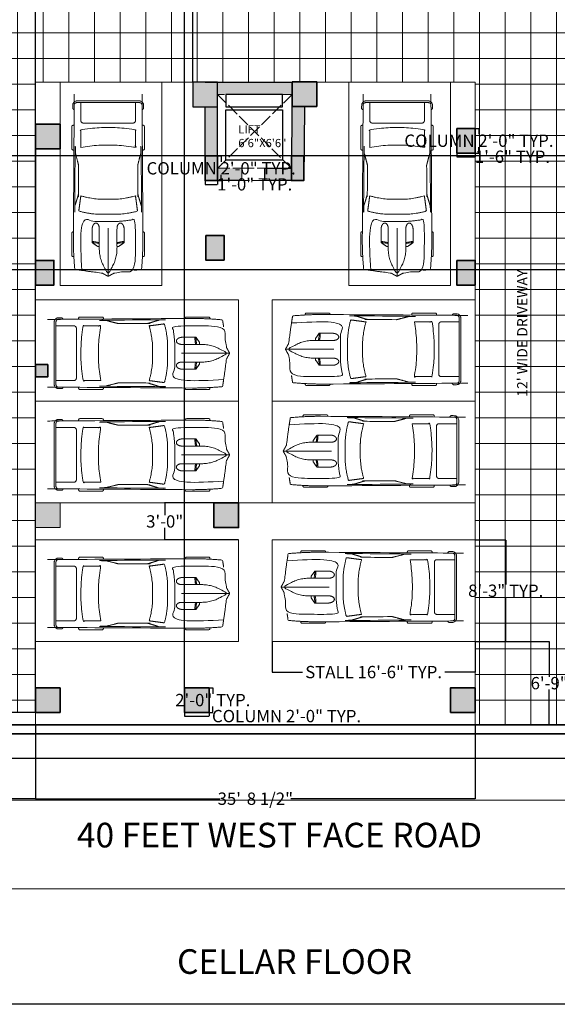
# Model space of a CAD drawing. Units: inches. Extents: x 48986 to 50522, y 132527 to 134098.
# Tile 2 of 4: x 49552 to 50076, y 132529 to 133488. Entities that reach past the tile are written whole.
import ezdxf

# ---------------------------------------------------------------- set-up
doc = ezdxf.new("R2010")
doc.units = ezdxf.units.IN
doc.header["$MEASUREMENT"] = 0
doc.linetypes.add('ACAD_ISO02W100', pattern=[15, 12, -3])
for name, color, linetype, lineweight in [('A-ANNO-DIMS', 2, 'Continuous', 18), ('A-ANNO-TEXT', 7, 'Continuous', 18), ('A-ANNO-TTLB', 7, 'Continuous', 25), ('A-AREA-IDEN', 7, 'Continuous', 18), ('A-COLS-PATT', 215, 'Continuous', 13), ('A-EQPM-VEHC', 8, 'Continuous', 13), ('A-FLOR-EVTR', 7, 'Continuous', 25), ('A-FLOR-PATT', 94, 'Continuous', 9), ('A-FLOR-PKNG', 140, 'Continuous', 18), ('A-WALL-PATT', 254, 'Continuous', 13), ('C-PROP', 160, 'Continuous', 25), ('C-ROAD', 7, 'Continuous', 18), ('COLUMNS', 211, 'Continuous', 35), ('lift', 7, 'ACAD_ISO02W100', 18), ('WALLS', 140, 'Continuous', 35)]:
    doc.layers.add(name, color=color, linetype=linetype, lineweight=lineweight)
doc.styles.get("Standard").update_dxf_attribs({"font": 'arial.ttf'})
doc.dimstyles.get("Standard").update_dxf_attribs({"dimtxt": 12, "dimasz": 0.18, "dimexe": 0.18, "dimexo": 0.0625, "dimgap": 0.09, "dimtad": 0, "dimtih": 1, "dimtoh": 1, "dimdec": 1, "dimzin": 0, "dimdsep": 46, "dimlunit": 3, "dimtxsty": 'Standard', "dimcen": 0.09, "dimadec": 0, "dimazin": 0, "dimtfac": 1, "dimtdec": 1, "dimtofl": 0, "dimtmove": 0, "dimatfit": 3, "dimfxl": 1, "dimtolj": 1, "dimtzin": 0, "dimarcsym": 0})

# ---------------------------------------------------------------- blocks, each defined once
blk = doc.blocks.new('CAR-SEDAN-PLAN')
for p, q in [((35.28, 177.53), (35.28, 130.65)), ((25.73, 8.37), (44.83, 8.37))]:
    blk.add_line(p, q)
for centre, major_axis, start_param, end_param in [((19.85, 164.65), (-24.87, 0), 1.564964, 1.848039), ((50.71, 164.65), (24.87, 0), 4.435146, 4.718221)]:
    blk.add_ellipse(centre, major_axis=major_axis, ratio=0.842304, start_param=start_param, end_param=end_param)
for points, weights, knots in [([(60.93, 171.77), (56.4, 172.48), (51.85, 173.06), (46.33, 173.7), (40.84, 174.57), (38.25, 176), (35.65, 177.44), (35.28, 177.64), (34.91, 177.44), (32.32, 176), (29.72, 174.57), (24.24, 173.7), (18.71, 173.06), (14.16, 172.48), (9.64, 171.77), (7.88, 146.82), (9.23, 121.85), (17.23, 123.66), (25.51, 124.08), (35.28, 124.08), (45.06, 124.08), (53.33, 123.66), (61.34, 121.85), (62.69, 146.82), (60.93, 171.77)], [1, 0.999861960732, 1, 0.999699858145, 1, 1, 1, 0.835952709181, 1, 1, 1, 0.999699858145, 1, 0.999861960732, 1, 0.998625728423, 1, 0.994860280211, 1, 1, 1, 0.994860280211, 1, 0.998625728423, 1], [0, 0, 0, 0.033232, 0.033232, 0.082234, 0.082234, 1.082234, 1.082234, 2.244094, 2.244094, 3.244094, 3.244094, 3.293097, 3.293097, 3.326328, 3.326328, 3.431193, 3.431193, 3.634055, 3.634055, 4.634055, 4.634055, 4.836917, 4.836917, 4.941783, 4.941783, 4.941783]), ([(43.91, 145.56), (47.31, 144.74), (50.86, 144.76), (50.86, 138.04), (50.86, 131.32), (50.59, 126.02), (47.38, 125.71), (44.17, 125.4), (43.91, 130.65), (43.91, 140.58), (43.91, 150.52), (43.91, 163.57), (35.28, 174.41), (26.66, 163.57), (26.66, 150.52), (26.66, 140.58), (26.66, 130.65), (26.39, 125.4), (23.18, 125.71), (19.97, 126.02), (19.71, 131.32), (19.71, 138.04), (19.71, 144.76), (23.25, 144.74), (26.66, 145.56)], [1, 0.990000279832, 1, 1, 1, 0.735618766318, 1, 0.735618766318, 1, 1, 1, 0.956755789522, 1, 0.956755789522, 1, 1, 1, 0.735618766318, 1, 0.735618766318, 1, 1, 1, 0.990000279832, 1], [0, 0, 0, 0.283075, 0.283075, 1.283075, 1.283075, 2.771508, 2.771508, 4.259942, 4.259942, 5.259942, 5.259942, 5.85026, 5.85026, 6.440579, 6.440579, 7.440579, 7.440579, 8.929012, 8.929012, 10.417446, 10.417446, 11.417446, 11.417446, 11.700521, 11.700521, 11.700521]), ([(9.64, 171.77), (6.18, 171.25), (2.75, 170.65), (1.43, 155.99), (1.38, 141.3)], [1, 0.999923835344, 1, 0.999337806115, 1], [0, 0, 0, 0.02468451, 0.02468451, 0.0974728, 0.0974728, 0.0974728]), ([(69.18, 141.3), (69.13, 155.99), (67.82, 170.65), (64.38, 171.25), (60.93, 171.77)], [1, 0.999337806115, 1, 0.999923835344, 1], [0, 0, 0, 0.07278829, 0.07278829, 0.0974728, 0.0974728, 0.0974728]), ([(1.87, 158.39), (1.61, 158.39), (1.35, 158.39), (0.79, 158.39), (0.4, 158.06), (0, 157.72), (0, 157.26), (0, 146.28), (0, 135.3), (0, 134.83), (0.4, 134.5), (0.79, 134.17), (1.35, 134.17), (1.35, 134.17), (1.36, 134.17)], [1, 1, 1, 0.923879532511, 1, 0.923879532511, 1, 1, 1, 0.923879532511, 1, 0.923879532511, 1, 1, 1], [0, 0, 0, 1, 1, 1.785398, 1.785398, 2.570796, 2.570796, 3.570796, 3.570796, 4.356194, 4.356194, 5.141593, 5.141593, 6.141593, 6.141593, 6.141593]), ([(69.2, 134.17), (69.21, 134.17), (69.22, 134.17), (69.77, 134.17), (70.17, 134.5), (70.56, 134.83), (70.56, 135.3), (70.56, 146.28), (70.56, 157.26), (70.56, 157.72), (70.17, 158.06), (69.77, 158.39), (69.22, 158.39), (68.96, 158.39), (68.7, 158.39)], [1, 1, 1, 0.923879532511, 1, 0.923879532511, 1, 1, 1, 0.923879532511, 1, 0.923879532511, 1, 1, 1], [0, 0, 0, 1, 1, 1.785398, 1.785398, 2.570796, 2.570796, 3.570796, 3.570796, 4.356194, 4.356194, 5.141593, 5.141593, 6.141593, 6.141593, 6.141593]), ([(26.66, 148.39), (25.91, 148.39), (25.16, 148.39), (24.92, 148.39), (24.74, 148.26), (22.22, 146.51), (19.71, 144.76)], [1, 1, 1, 0.940892222322, 1, 1, 1], [0, 0, 0, 1, 1, 1.691083, 1.691083, 2.691083, 2.691083, 2.691083]), ([(50.86, 144.76), (48.34, 146.51), (45.83, 148.26), (45.64, 148.39), (45.4, 148.39), (44.65, 148.39), (43.91, 148.39)], [1, 1, 1, 0.940892222322, 1, 1, 1], [0, 0, 0, 1, 1, 1.691083, 1.691083, 2.691083, 2.691083, 2.691083]), ([(1.38, 141.68), (1.17, 76.13), (2.21, 10.6), (2.24, 8.37), (4.89, 8.37), (35.28, 8.37), (65.67, 8.37), (68.32, 8.37), (68.36, 10.6), (69.4, 76.13), (69.18, 141.68)], [1, 0.999967219517, 1, 0.711827418646, 1, 1, 1, 0.711827418646, 1, 0.999967219517, 1], [0, 0, 0, 0.016194, 0.016194, 1.573593, 1.573593, 2.573593, 2.573593, 4.130993, 4.130993, 4.147187, 4.147187, 4.147187]), ([(6.45, 69.32), (4.72, 62.5), (2.98, 55.69), (2.73, 82.7), (2.7, 109.71), (4.53, 103.71), (6.37, 97.71), (6.33, 83.51), (6.45, 69.32)], [1, 1, 1, 0.999994429546, 1, 1, 1, 0.999987377106, 1], [0, 0, 0, 1, 1, 1.006676, 1.006676, 2.006676, 2.006676, 2.016725, 2.016725, 2.016725]), ([(61.91, 99.15), (52.72, 101.89), (42.99, 102.47), (35.28, 102.47), (27.57, 102.47), (17.85, 101.89), (8.66, 99.15), (7.66, 106.57), (6.67, 114), (15.95, 116.64), (25.73, 117.16), (35.28, 117.16), (44.83, 117.16), (54.61, 116.64), (63.89, 114), (62.9, 106.57), (61.91, 99.15)], [1, 0.991000078903, 1, 1, 1, 0.991000078903, 1, 1, 1, 0.991394232237, 1, 1, 1, 0.991394232237, 1, 1, 1], [0, 0, 0, 0.268529, 0.268529, 1.268529, 1.268529, 1.537057, 1.537057, 2.537057, 2.537057, 2.799631, 2.799631, 3.799631, 3.799631, 4.062205, 4.062205, 5.062205, 5.062205, 5.062205]), ([(64.11, 69.32), (64.24, 83.51), (64.2, 97.71), (66.03, 103.71), (67.87, 109.71), (67.83, 82.7), (67.58, 55.69), (65.85, 62.5), (64.11, 69.32)], [1, 0.999987377106, 1, 1, 1, 0.999994429546, 1, 1, 1], [0, 0, 0, 0.010049, 0.010049, 1.010049, 1.010049, 1.016725, 1.016725, 2.016725, 2.016725, 2.016725]), ([(1.65, 54.65), (1.5, 54.65), (1.35, 54.65), (0, 54.65), (0, 53.52), (0, 42.54), (0, 31.57), (0, 30.44), (1.35, 30.44), (1.63, 30.44), (1.92, 30.44)], [1, 1, 1, 0.707106781187, 1, 1, 1, 0.707106781187, 1, 1, 1], [0, 0, 0, 1, 1, 2.570796, 2.570796, 3.570796, 3.570796, 5.141593, 5.141593, 6.141593, 6.141593, 6.141593]), ([(61.91, 51.96), (35.28, 47.39), (8.66, 51.96), (8.66, 43.42), (8.66, 34.88), (35.28, 30.31), (61.91, 34.88), (61.91, 43.42), (61.91, 51.96)], [1, 0.979868494456, 1, 1, 1, 0.979868494456, 1, 1, 1], [0, 0, 0, 0.401989, 0.401989, 1.401989, 1.401989, 1.803978, 1.803978, 2.803978, 2.803978, 2.803978]), ([(68.64, 30.44), (68.93, 30.44), (69.22, 30.44), (69.77, 30.44), (70.17, 30.77), (70.56, 31.1), (70.56, 31.57), (70.56, 42.54), (70.56, 53.52), (70.56, 53.99), (70.17, 54.32), (69.77, 54.65), (69.22, 54.65), (69.07, 54.65), (68.91, 54.65)], [1, 1, 1, 0.923879532511, 1, 0.923879532511, 1, 1, 1, 0.923879532511, 1, 0.923879532511, 1, 1, 1], [0, 0, 0, 1, 1, 1.785398, 1.785398, 2.570796, 2.570796, 3.570796, 3.570796, 4.356194, 4.356194, 5.141593, 5.141593, 6.141593, 6.141593, 6.141593]), ([(61.91, 8.37), (61.91, 17.2), (61.91, 26.03), (61.91, 28.29), (59.22, 28.29), (35.28, 28.29), (11.34, 28.29), (8.66, 28.29), (8.66, 26.03), (8.66, 17.2), (8.66, 8.37)], [1, 1, 1, 0.707106781187, 1, 1, 1, 0.707106781187, 1, 1, 1], [0, 0, 0, 1, 1, 2.570796, 2.570796, 3.570796, 3.570796, 5.141593, 5.141593, 6.141593, 6.141593, 6.141593]), ([(2.14, 15.28), (0.74, 14.89), (0.76, 13.65), (0.78, 12.11), (0.81, 10.58), (0.87, 6.62), (5.56, 6.62), (35.28, 6.62), (65, 6.62), (69.7, 6.62), (69.76, 10.58), (69.78, 12.11), (69.81, 13.65), (69.83, 14.89), (68.43, 15.28)], [1, 0.807168985933, 1, 0.999999981995, 1, 0.711827418646, 1, 1, 1, 0.711827418646, 1, 0.999999981995, 1, 0.807168985459, 1], [0, 0, 0, 1.262912, 1.262912, 1.263291, 1.263291, 2.82069, 2.82069, 3.82069, 3.82069, 5.37809, 5.37809, 5.378469, 5.378469, 6.641381, 6.641381, 6.641381])]:
    blk.add_rational_spline(points, weights, degree=2, knots=knots)
blk = doc.blocks.new('PARKING-STALL-99X198')
blk.add_lwpolyline([(198, 0), (198, 99), (0, 99), (0, 0)], close=True)
blk = doc.blocks.new('COL-24X24')
blk.add_lwpolyline([(24, 24), (24, 0), (0, 0), (0, 24)], close=True)
blk = doc.blocks.new('COL-18X24')
blk.add_lwpolyline([(0, 24), (0, 12.32), (0, 0), (18, 0), (18, 24)], close=True)
blk = doc.blocks.new('COL-12X24')
blk.add_lwpolyline([(0, 24), (12, 24), (12, 0), (0, 0)], close=True)
blk = doc.blocks.new('*D13')
at = {"layer": 'A-ANNO-DIMS', "color": 0, "lineweight": -2, "transparency": 16777216}
for p, q in [((49797.88, 132881.98), (49797.88, 132852.17)), ((49995.88, 132881.98), (49995.88, 132852.17)), ((49798.06, 132852.35), (49827.63, 132852.35)), ((49995.7, 132852.35), (49966.13, 132852.35))]:
    blk.add_line(p, q, dxfattribs=at)
at = {"layer": 'A-ANNO-DIMS', "color": 0, "transparency": 16777216}
for points in [[(49798.06, 132852.38), (49798.06, 132852.32), (49797.88, 132852.35)], [(49995.7, 132852.38), (49995.7, 132852.32), (49995.88, 132852.35)]]:
    blk.add_solid(points, dxfattribs=at)
at = {"layer": 'Defpoints', "color": 0, "transparency": 16777216}
for p in [(49797.88, 132882.05), (49995.88, 132882.05), (49995.88, 132852.35)]:
    blk.add_point(p, dxfattribs=at)
at = {"layer": 'A-ANNO-DIMS', "color": 0, "transparency": 16777216, "insert": (49896.88, 132852.35), "char_height": 12, "attachment_point": 5}
blk.add_mtext('\\A1;STALL 16\'-6" TYP.', dxfattribs=at)
blk = doc.blocks.new('*D14')
at = {"layer": 'A-ANNO-DIMS', "color": 0, "lineweight": -2, "transparency": 16777216}
for p, q in [((49995.94, 132981.05), (50025.76, 132981.05)), ((50025.58, 132980.87), (50025.58, 132937.77)), ((50025.58, 132882.23), (50025.58, 132925.32)), ((49995.94, 132882.05), (50025.76, 132882.05))]:
    blk.add_line(p, q, dxfattribs=at)
at = {"layer": 'A-ANNO-DIMS', "color": 0, "transparency": 16777216}
for points in [[(50025.55, 132980.87), (50025.61, 132980.87), (50025.58, 132981.05)], [(50025.55, 132882.23), (50025.61, 132882.23), (50025.58, 132882.05)]]:
    blk.add_solid(points, dxfattribs=at)
at = {"layer": 'Defpoints', "color": 0, "transparency": 16777216}
for p in [(49995.88, 132981.05), (50025.58, 132981.05), (49995.88, 132882.05)]:
    blk.add_point(p, dxfattribs=at)
at = {"layer": 'A-ANNO-DIMS', "color": 0, "transparency": 16777216, "insert": (50025.58, 132931.55), "char_height": 12, "attachment_point": 5}
blk.add_mtext('\\A1;8\'-3" TYP.', dxfattribs=at)
blk = doc.blocks.new('*D15')
at = {"layer": 'A-ANNO-DIMS', "color": 0, "lineweight": -2, "transparency": 16777216}
for p, q in [((49712.57, 132812.99), (49712.57, 132809.28)), ((49712.75, 132809.46), (49736.39, 132809.46)), ((49736.57, 132812.99), (49736.57, 132809.28)), ((49736.57, 132809.46), (49736.75, 132809.46))]:
    blk.add_line(p, q, dxfattribs=at)
at = {"layer": 'A-ANNO-DIMS', "color": 0, "transparency": 16777216}
for points in [[(49712.75, 132809.49), (49712.75, 132809.43), (49712.57, 132809.46)], [(49736.39, 132809.49), (49736.39, 132809.43), (49736.57, 132809.46)]]:
    blk.add_solid(points, dxfattribs=at)
at = {"layer": 'Defpoints', "color": 0, "transparency": 16777216}
for p in [(49712.57, 132813.06), (49736.57, 132813.06), (49736.57, 132809.46)]:
    blk.add_point(p, dxfattribs=at)
at = {"layer": 'A-ANNO-DIMS', "color": 0, "transparency": 16777216, "insert": (49812, 132809.46), "char_height": 12, "attachment_point": 5}
blk.add_mtext('\\A1;COLUMN 2\'-0" TYP.', dxfattribs=at)
blk = doc.blocks.new('*D16')
at = {"layer": 'A-ANNO-DIMS', "color": 0, "lineweight": -2, "transparency": 16777216}
for p, q in [((49736.63, 132837.06), (49740.35, 132837.06)), ((49740.17, 132836.88), (49740.17, 132831.27)), ((49740.17, 132813.24), (49740.17, 132818.84)), ((49736.63, 132813.06), (49740.35, 132813.06))]:
    blk.add_line(p, q, dxfattribs=at)
at = {"layer": 'A-ANNO-DIMS', "color": 0, "transparency": 16777216}
for points in [[(49740.14, 132836.88), (49740.2, 132836.88), (49740.17, 132837.06)], [(49740.14, 132813.24), (49740.2, 132813.24), (49740.17, 132813.06)]]:
    blk.add_solid(points, dxfattribs=at)
at = {"layer": 'Defpoints', "color": 0, "transparency": 16777216}
for p in [(49736.57, 132837.06), (49740.17, 132837.06), (49736.57, 132813.06)]:
    blk.add_point(p, dxfattribs=at)
at = {"layer": 'A-ANNO-DIMS', "color": 0, "transparency": 16777216, "insert": (49740.17, 132825.06), "char_height": 12, "attachment_point": 5}
blk.add_mtext('\\A1;2\'-0" TYP.', dxfattribs=at)
blk = doc.blocks.new('*D17')
at = {"layer": 'A-ANNO-DIMS', "color": 0, "lineweight": -2, "transparency": 16777216}
for p, q in [((49995.94, 133381.91), (49999.66, 133381.91)), ((49999.48, 133381.73), (49999.48, 133376.2)), ((49999.48, 133358.09), (49999.48, 133363.61)), ((49995.94, 133357.91), (49999.66, 133357.91))]:
    blk.add_line(p, q, dxfattribs=at)
at = {"layer": 'A-ANNO-DIMS', "color": 0, "transparency": 16777216}
for points in [[(49999.45, 133381.73), (49999.51, 133381.73), (49999.48, 133381.91)], [(49999.45, 133358.09), (49999.51, 133358.09), (49999.48, 133357.91)]]:
    blk.add_solid(points, dxfattribs=at)
at = {"layer": 'Defpoints', "color": 0, "transparency": 16777216}
for p in [(49995.88, 133381.91), (49999.48, 133381.91), (49995.88, 133357.91)]:
    blk.add_point(p, dxfattribs=at)
at = {"layer": 'A-ANNO-DIMS', "color": 0, "transparency": 16777216, "insert": (49999.48, 133369.91), "char_height": 12, "attachment_point": 5}
blk.add_mtext('\\A1;COLUMN 2\'-0" TYP.', dxfattribs=at)
blk = doc.blocks.new('*D18')
at = {"layer": 'A-ANNO-DIMS', "color": 0, "lineweight": -2, "transparency": 16777216}
for p, q in [((49977.88, 133357.84), (49977.88, 133354.13)), ((49978.06, 133354.31), (49995.7, 133354.31)), ((49995.88, 133357.84), (49995.88, 133354.13)), ((49995.88, 133354.31), (49996.06, 133354.31))]:
    blk.add_line(p, q, dxfattribs=at)
at = {"layer": 'A-ANNO-DIMS', "color": 0, "transparency": 16777216}
for points in [[(49978.06, 133354.34), (49978.06, 133354.28), (49977.88, 133354.31)], [(49995.7, 133354.34), (49995.7, 133354.28), (49995.88, 133354.31)]]:
    blk.add_solid(points, dxfattribs=at)
at = {"layer": 'Defpoints', "color": 0, "transparency": 16777216}
for p in [(49977.88, 133357.91), (49995.88, 133357.91), (49995.88, 133354.31)]:
    blk.add_point(p, dxfattribs=at)
at = {"layer": 'A-ANNO-DIMS', "color": 0, "transparency": 16777216, "insert": (50032.16, 133354.31), "char_height": 12, "attachment_point": 5}
blk.add_mtext('\\A1;1\'-6" TYP.', dxfattribs=at)
blk = doc.blocks.new('*D21')
at = {"layer": 'A-ANNO-DIMS', "color": 0, "lineweight": -2, "transparency": 16777216}
for p, q in [((49744.77, 133355), (49748.49, 133355)), ((49748.31, 133354.82), (49748.31, 133349.3)), ((49748.31, 133331.18), (49748.31, 133336.7)), ((49744.77, 133331), (49748.49, 133331))]:
    blk.add_line(p, q, dxfattribs=at)
at = {"layer": 'A-ANNO-DIMS', "color": 0, "transparency": 16777216}
for points in [[(49748.28, 133354.82), (49748.34, 133354.82), (49748.31, 133355)], [(49748.28, 133331.18), (49748.34, 133331.18), (49748.31, 133331)]]:
    blk.add_solid(points, dxfattribs=at)
at = {"layer": 'Defpoints', "color": 0, "transparency": 16777216}
for p in [(49744.71, 133355), (49748.31, 133355), (49744.71, 133331)]:
    blk.add_point(p, dxfattribs=at)
at = {"layer": 'A-ANNO-DIMS', "color": 0, "transparency": 16777216, "insert": (49748.31, 133343), "char_height": 12, "attachment_point": 5}
blk.add_mtext('\\A1;COLUMN 2\'-0" TYP.', dxfattribs=at)
blk = doc.blocks.new('*D22')
at = {"layer": 'A-ANNO-DIMS', "color": 0, "lineweight": -2, "transparency": 16777216}
for p, q in [((49732.71, 133330.93), (49732.71, 133327.22)), ((49732.89, 133327.4), (49744.53, 133327.4)), ((49744.71, 133330.93), (49744.71, 133327.22)), ((49744.71, 133327.4), (49744.89, 133327.4))]:
    blk.add_line(p, q, dxfattribs=at)
at = {"layer": 'A-ANNO-DIMS', "color": 0, "transparency": 16777216}
for points in [[(49732.89, 133327.43), (49732.89, 133327.37), (49732.71, 133327.4)], [(49744.53, 133327.43), (49744.53, 133327.37), (49744.71, 133327.4)]]:
    blk.add_solid(points, dxfattribs=at)
at = {"layer": 'Defpoints', "color": 0, "transparency": 16777216}
for p in [(49732.71, 133331), (49744.71, 133331), (49744.71, 133327.4)]:
    blk.add_point(p, dxfattribs=at)
at = {"layer": 'A-ANNO-DIMS', "color": 0, "transparency": 16777216, "insert": (49780.99, 133327.4), "char_height": 12, "attachment_point": 5}
blk.add_mtext('\\A1;1\'-0" TYP.', dxfattribs=at)
blk = doc.blocks.new('*D27')
at = {"layer": 'A-ANNO-DIMS', "color": 0, "lineweight": -2, "transparency": 16777216}
for p, q in [((49221.79, 132800.99), (49221.79, 132728.83)), ((49567.36, 132800.99), (49567.36, 132728.83)), ((49221.97, 132729.01), (49359.79, 132729.01)), ((49567.18, 132729.01), (49429.36, 132729.01))]:
    blk.add_line(p, q, dxfattribs=at)
at = {"layer": 'A-ANNO-DIMS', "color": 0, "transparency": 16777216}
for points in [[(49221.97, 132729.04), (49221.97, 132728.98), (49221.79, 132729.01)], [(49567.18, 132729.04), (49567.18, 132728.98), (49567.36, 132729.01)]]:
    blk.add_solid(points, dxfattribs=at)
at = {"layer": 'Defpoints', "color": 0, "transparency": 16777216}
for p in [(49221.79, 132801.06), (49567.36, 132801.06), (49221.79, 132729.01)]:
    blk.add_point(p, dxfattribs=at)
at = {"layer": 'A-ANNO-DIMS', "color": 0, "transparency": 16777216, "insert": (49394.57, 132729.01), "char_height": 12, "attachment_point": 5}
blk.add_mtext('\\A1;28\'-9 1/2"', dxfattribs=at)
blk = doc.blocks.new('*D28')
at = {"layer": 'A-ANNO-DIMS', "color": 0, "lineweight": -2, "transparency": 16777216}
for p, q in [((49567.36, 132800.99), (49567.36, 132728.83)), ((49995.88, 132800.99), (49995.88, 132728.83)), ((49567.54, 132729.01), (49746.94, 132729.01)), ((49995.7, 132729.01), (49816.3, 132729.01))]:
    blk.add_line(p, q, dxfattribs=at)
at = {"layer": 'A-ANNO-DIMS', "color": 0, "transparency": 16777216}
for points in [[(49567.54, 132729.04), (49567.54, 132728.98), (49567.36, 132729.01)], [(49995.7, 132729.04), (49995.7, 132728.98), (49995.88, 132729.01)]]:
    blk.add_solid(points, dxfattribs=at)
at = {"layer": 'Defpoints', "color": 0, "transparency": 16777216}
for p in [(49567.36, 132801.06), (49995.88, 132801.06), (49567.36, 132729.01)]:
    blk.add_point(p, dxfattribs=at)
at = {"layer": 'A-ANNO-DIMS', "color": 0, "transparency": 16777216, "insert": (49781.62, 132729.01), "char_height": 12, "attachment_point": 5}
blk.add_mtext('\\A1;35\'-8 1/2"', dxfattribs=at)
blk = doc.blocks.new('*D30')
at = {"layer": 'A-ANNO-DIMS', "color": 0, "lineweight": -2, "transparency": 16777216}
for p, q in [((50139.82, 133355.06), (49029.36, 133355.06)), ((49029.54, 133354.88), (49029.54, 133305.73)), ((49029.54, 133244.15), (49029.54, 133293.29)), ((50139.82, 133243.97), (49029.36, 133243.97))]:
    blk.add_line(p, q, dxfattribs=at)
at = {"layer": 'A-ANNO-DIMS', "color": 0, "transparency": 16777216}
for points in [[(49029.51, 133354.88), (49029.57, 133354.88), (49029.54, 133355.06)], [(49029.51, 133244.15), (49029.57, 133244.15), (49029.54, 133243.97)]]:
    blk.add_solid(points, dxfattribs=at)
at = {"layer": 'Defpoints', "color": 0, "transparency": 16777216}
for p in [(49029.54, 133355.06), (50139.88, 133355.06), (50139.88, 133243.97)]:
    blk.add_point(p, dxfattribs=at)
at = {"layer": 'A-ANNO-DIMS', "color": 0, "transparency": 16777216, "insert": (49029.54, 133299.51), "char_height": 12, "attachment_point": 5}
blk.add_mtext('\\A1;9\'-3"', dxfattribs=at)
blk = doc.blocks.new('*D36')
at = {"layer": 'A-ANNO-DIMS', "color": 0, "lineweight": -2, "transparency": 16777216}
for p, q in [((49567.36, 133427.06), (49567.36, 133901.29)), ((49567.54, 133901.11), (49609.92, 133901.11)), ((49720.53, 133901.11), (49678.15, 133901.11)), ((49720.71, 133427.06), (49720.71, 133901.29))]:
    blk.add_line(p, q, dxfattribs=at)
at = {"layer": 'A-ANNO-DIMS', "color": 0, "transparency": 16777216}
for points in [[(49567.54, 133901.14), (49567.54, 133901.08), (49567.36, 133901.11)], [(49720.53, 133901.14), (49720.53, 133901.08), (49720.71, 133901.11)]]:
    blk.add_solid(points, dxfattribs=at)
at = {"layer": 'Defpoints', "color": 0, "transparency": 16777216}
for p in [(49720.71, 133901.11), (49567.36, 133426.99), (49720.71, 133426.99)]:
    blk.add_point(p, dxfattribs=at)
at = {"layer": 'A-ANNO-DIMS', "color": 0, "transparency": 16777216, "insert": (49644.03, 133901.11), "char_height": 12, "attachment_point": 5}
blk.add_mtext('\\A1;12\'-9 1/2"', dxfattribs=at)
blk = doc.blocks.new('*D38')
at = {"layer": 'A-ANNO-DIMS', "color": 0, "lineweight": -2, "transparency": 16777216}
for p, q in [((49995.94, 132882.05), (50068.11, 132882.05)), ((50067.93, 132881.87), (50067.93, 132847.77)), ((50067.93, 132801.24), (50067.93, 132835.33)), ((49995.94, 132801.06), (50068.11, 132801.06))]:
    blk.add_line(p, q, dxfattribs=at)
at = {"layer": 'A-ANNO-DIMS', "color": 0, "transparency": 16777216}
for points in [[(50067.9, 132881.87), (50067.96, 132881.87), (50067.93, 132882.05)], [(50067.9, 132801.24), (50067.96, 132801.24), (50067.93, 132801.06)]]:
    blk.add_solid(points, dxfattribs=at)
at = {"layer": 'Defpoints', "color": 0, "transparency": 16777216}
for p in [(49995.88, 132882.05), (49995.88, 132801.06), (50067.93, 132801.06)]:
    blk.add_point(p, dxfattribs=at)
at = {"layer": 'A-ANNO-DIMS', "color": 0, "transparency": 16777216, "insert": (50067.93, 132841.55), "char_height": 12, "attachment_point": 5}
blk.add_mtext('\\A1;6\'-9"', dxfattribs=at)
blk = doc.blocks.new('*D39')
at = {"layer": 'A-ANNO-DIMS', "color": 0, "lineweight": -2, "transparency": 16777216}
for p, q in [((49765.3, 133017.05), (49693.13, 133017.05)), ((49693.31, 133016.87), (49693.31, 133005.27)), ((49693.31, 132981.23), (49693.31, 132992.82)), ((49765.3, 132981.05), (49693.13, 132981.05))]:
    blk.add_line(p, q, dxfattribs=at)
at = {"layer": 'A-ANNO-DIMS', "color": 0, "transparency": 16777216}
for points in [[(49693.28, 133016.87), (49693.34, 133016.87), (49693.31, 133017.05)], [(49693.28, 132981.23), (49693.34, 132981.23), (49693.31, 132981.05)]]:
    blk.add_solid(points, dxfattribs=at)
at = {"layer": 'Defpoints', "color": 0, "transparency": 16777216}
for p in [(49693.31, 133017.05), (49765.36, 133017.05), (49765.36, 132981.05)]:
    blk.add_point(p, dxfattribs=at)
at = {"layer": 'A-ANNO-DIMS', "color": 0, "transparency": 16777216, "insert": (49693.31, 132999.05), "char_height": 12, "attachment_point": 5}
blk.add_mtext('\\A1;3\'-0"', dxfattribs=at)
blk = doc.blocks.new('*D44')
at = {"layer": 'A-ANNO-DIMS', "color": 0, "lineweight": -2, "transparency": 16777216}
for p, q in [((49567.36, 132837.12), (49567.36, 133901.29)), ((49567.54, 133901.11), (49619.83, 133901.11)), ((49712.39, 133901.11), (49660.1, 133901.11)), ((49712.57, 132837.12), (49712.57, 133901.29))]:
    blk.add_line(p, q, dxfattribs=at)
at = {"layer": 'A-ANNO-DIMS', "color": 0, "transparency": 16777216}
for points in [[(49567.54, 133901.14), (49567.54, 133901.08), (49567.36, 133901.11)], [(49712.39, 133901.14), (49712.39, 133901.08), (49712.57, 133901.11)]]:
    blk.add_solid(points, dxfattribs=at)
at = {"layer": 'Defpoints', "color": 0, "transparency": 16777216}
for p in [(49712.57, 133901.11), (49567.36, 132837.06), (49712.57, 132837.06)]:
    blk.add_point(p, dxfattribs=at)
at = {"layer": 'A-ANNO-DIMS', "color": 0, "transparency": 16777216, "insert": (49639.96, 133901.11), "char_height": 12, "attachment_point": 5}
blk.add_mtext('\\A1;12\'-1"', dxfattribs=at)
blk = doc.blocks.new('*D45')
at = {"layer": 'A-ANNO-DIMS', "color": 0, "lineweight": -2, "transparency": 16777216}
for p, q in [((49567.3, 132813.06), (49495.13, 132813.06)), ((49495.31, 132813.06), (49495.31, 132813.24)), ((49495.31, 132813.24), (49495.49, 132813.24)), ((49495.31, 132801.24), (49495.31, 132812.88)), ((49567.3, 132801.06), (49495.13, 132801.06))]:
    blk.add_line(p, q, dxfattribs=at)
at = {"layer": 'A-ANNO-DIMS', "color": 0, "transparency": 16777216}
for points in [[(49495.28, 132812.88), (49495.34, 132812.88), (49495.31, 132813.06)], [(49495.28, 132801.24), (49495.34, 132801.24), (49495.31, 132801.06)]]:
    blk.add_solid(points, dxfattribs=at)
at = {"layer": 'Defpoints', "color": 0, "transparency": 16777216}
for p in [(49495.31, 132813.06), (49567.36, 132813.06), (49567.36, 132801.06)]:
    blk.add_point(p, dxfattribs=at)
at = {"layer": 'A-ANNO-DIMS', "color": 0, "transparency": 16777216, "insert": (49510.96, 132813.24), "char_height": 12, "attachment_point": 5}
blk.add_mtext('\\A1;1\'-0"', dxfattribs=at)

msp = doc.modelspace()

# ---------------------------------------------------------------- hatches: boundary and pattern name
at = {"layer": 'A-COLS-PATT'}
h = msp.add_hatch(color=256, dxfattribs=at)
h.dxf.hatch_style = 1
h.paths.add_polyline_path([(49744.71, 133426.99), (49720.71, 133426.99), (49720.71, 133402.99), (49744.71, 133402.99)])
h.paths.add_polyline_path([(49841.62, 133427.11), (49817.62, 133427.11), (49817.62, 133403.11), (49841.62, 133403.11)])
h.paths.add_polyline_path([(49828.71, 133355), (49816.71, 133355), (49816.71, 133331), (49828.71, 133331)])
h.paths.add_polyline_path([(49744.71, 133355), (49732.71, 133355), (49732.71, 133331), (49744.71, 133331)])
h = msp.add_hatch(color=256, dxfattribs=at)
h.dxf.hatch_style = 1
h.paths.add_polyline_path([(49591.36, 133385.98), (49567.36, 133385.98), (49567.36, 133361.98), (49591.36, 133361.98)])
h.paths.add_polyline_path([(49585.36, 133253.31), (49567.36, 133253.31), (49567.36, 133241.64), (49567.36, 133229.31), (49585.36, 133229.31)])
h.paths.add_polyline_path([(49751.22, 133277.58), (49733.22, 133277.58), (49733.22, 133265.9), (49733.22, 133253.58), (49751.22, 133253.58)])
h.paths.add_polyline_path([(49995.88, 133381.91), (49977.88, 133381.91), (49977.88, 133370.23), (49977.88, 133357.91), (49995.88, 133357.91)])
h.paths.add_polyline_path([(49995.88, 133253.24), (49977.88, 133253.24), (49977.88, 133241.56), (49977.88, 133229.24), (49995.88, 133229.24)])
h.paths.add_polyline_path([(49579.36, 133151.77), (49567.36, 133151.77), (49567.36, 133139.77), (49579.36, 133139.77)])
h.paths.add_polyline_path([(49591.36, 133017.05), (49567.36, 133017.05), (49567.36, 132993.05), (49591.36, 132993.05)])
h.paths.add_polyline_path([(49765.32, 133017.05), (49741.32, 133017.05), (49741.32, 132993.05), (49765.32, 132993.05)])
h.paths.add_polyline_path([(49591.36, 132837.06), (49567.36, 132837.06), (49567.36, 132813.06), (49591.36, 132813.06)])
h.paths.add_polyline_path([(49736.57, 132837.06), (49712.57, 132837.06), (49712.57, 132813.06), (49736.57, 132813.06)])
h.paths.add_polyline_path([(49995.88, 132837.06), (49971.88, 132837.06), (49971.88, 132813.06), (49995.88, 132813.06)])
at = {"layer": 'A-FLOR-PATT'}
h = msp.add_hatch(dxfattribs=at)
h.set_pattern_fill('NET', color=256, scale=200)
h.paths.add_polyline_path([(50323.33, 133597.94), (50298.79, 133598.06), (50199.79, 133598.06), (49957.56, 133598.06), (49597.63, 133598.06), (49221.79, 133598.06), (49221.79, 132801.06), (49253.29, 132801.06), (49253.29, 132832.63), (49251.14, 132832.63), (49251.14, 132842.53), (49253.29, 132842.53), (49253.29, 132956.08), (49251.14, 132956.08), (49251.14, 132965.97), (49253.29, 132965.97), (49253.29, 133105.3), (49251.14, 133105.3), (49251.14, 133115.2), (49253.29, 133115.2), (49253.29, 133143.75), (49253.29, 133153.65), (49253.29, 133244.43), (49251.14, 133244.43), (49251.14, 133254.33), (49253.29, 133254.33), (49253.29, 133283.54), (49253.29, 133293.44), (49253.29, 133335.08), (49251.14, 133335.08), (49248.66, 133335.08), (49248.66, 133344.97), (49251.14, 133344.97), (49253.29, 133344.97), (49253.29, 133387.65), (49253.29, 133397.55), (49253.29, 133425.06), (49253.29, 133426.99), (49420.79, 133426.99), (49423.36, 133426.99), (49423.36, 133344.97), (49425.09, 133344.97), (49425.09, 133335.08), (49423.36, 133335.08), (49423.36, 132813.06), (49567.36, 132813.06), (49567.36, 133229.31), (49567.36, 133241.64), (49567.36, 133265.64), (49567.36, 133335.08), (49567.36, 133344.97), (49567.36, 133361.98), (49567.36, 133385.98), (49567.36, 133426.99), (49591.36, 133426.99), (49690.36, 133426.99), (49817.62, 133426.99), (49817.62, 133427.11), (49841.62, 133427.11), (49995.88, 133426.99), (49995.88, 132801.06), (50139.88, 132801.06), (50139.88, 133259.08, -0.361241), (50136.6, 133263.03, -0.361241), (50139.88, 133266.99), (50139.88, 133448.06), (50303.12, 133448.06), (50303.12, 133472.06), (50323.33, 133472.06)])
at = {"layer": 'A-WALL-PATT'}
h = msp.add_hatch(color=256, dxfattribs=at)
h.dxf.hatch_style = 1
h.paths.add_polyline_path([(49817.62, 133426.99), (49781.62, 133426.99), (49744.71, 133426.99), (49744.71, 133414.99), (49781.62, 133414.99), (49817.51, 133414.99)])
h.paths.add_polyline_path([(49744.71, 133402.99), (49732.71, 133402.99), (49732.71, 133355), (49744.71, 133355)])
h.paths.add_polyline_path([(49829.39, 133403.11), (49817.62, 133403.11), (49817.62, 133414.99), (49817.51, 133414.99), (49816.94, 133355), (49828.71, 133355), (49828.71, 133331)])
h.paths.add_polyline_path([(49816.71, 133343), (49790.8, 133343), (49790.8, 133331), (49816.71, 133331)])
h.paths.add_polyline_path([(49768.42, 133343), (49744.71, 133343), (49744.71, 133331), (49768.42, 133331)])

# ---------------------------------------------------------------- linework, layer by layer
at = {"layer": 'A-ANNO-TTLB'}
msp.add_lwpolyline([(48985.99, 134098.01), (50521.96, 134098.01), (50521.96, 132528.75), (48985.99, 132528.75)], close=True, dxfattribs=at)
at = {"layer": 'A-FLOR-EVTR'}
msp.add_line((49817.62, 133427.11), (49816.94, 133355), dxfattribs=at)
for points in [[(49744.71, 133331), (49744.71, 133426.99), (49720.71, 133426.99), (49720.71, 133402.99), (49744.71, 133402.99), (49744.71, 133426.99)], [(49732.71, 133426.99), (49781.62, 133426.99), (49817.62, 133426.99)], [(49768.42, 133331), (49732.71, 133331), (49732.71, 133402.99)], [(49752.87, 133400.07), (49808.17, 133400.07), (49808.17, 133350.96), (49752.89, 133350.96), (49752.89, 133400.07)], [(49829.39, 133403.11), (49828.71, 133331), (49790.8, 133331), (49790.8, 133343), (49816.82, 133343)]]:
    msp.add_lwpolyline(points, dxfattribs=at)
msp.add_lwpolyline([(49808.17, 133402.99), (49808.17, 133414.99), (49752.89, 133414.99), (49752.89, 133406.75), (49752.89, 133402.99), (49753.5, 133402.99)], close=True, dxfattribs=at)
at = {"layer": 'A-FLOR-PKNG'}
for p, q in [((49567.36, 133426.99), (49567.36, 133385.98)), ((49567.36, 132936.06), (49567.36, 132972.06)), ((49567.36, 132882.05), (49765.36, 132882.05)), ((49995.88, 132882.05), (49797.88, 132882.05)), ((49797.88, 132882.05), (49881.53, 132882.05))]:
    msp.add_line(p, q, dxfattribs=at)
for points in [[(49591.36, 133322.53), (49591.36, 133228.99), (49591.36, 133426.99), (49567.36, 133426.99), (49995.88, 133426.99), (49971.88, 133426.99), (49971.88, 133228.99)], [(49995.88, 133426.99), (49995.88, 132801.06), (49995.88, 132837.06)], [(49567.36, 132801.06), (49567.36, 132801.06), (49567.36, 133229.31)], [(49765.36, 133017.05), (49567.36, 133017.05), (49591.36, 133017.05), (49591.36, 132993.05), (49567.36, 132993.05), (49567.36, 133017.05), (49765.36, 133017.05), (49765.36, 133116.05), (49765.36, 133215.05), (49567.36, 133215.05), (49567.36, 133116.05)], [(49765.36, 133116.05), (49567.36, 133116.05), (49567.36, 133017.05), (49765.36, 133017.05), (49720.31, 133017.05), (49995.88, 133017.05), (49797.88, 133017.05), (49797.88, 133116.05), (49995.88, 133116.05), (49797.88, 133116.05), (49797.88, 133215.05), (49995.88, 133215.05), (49995.88, 133116.05), (49995.88, 133017.05), (49797.88, 133017.05), (49881.53, 133017.05)], [(49567.36, 132837.06), (49567.36, 132801.06), (49567.36, 132813.06), (49423.36, 132813.06)]]:
    msp.add_lwpolyline(points, dxfattribs=at)
msp.add_lwpolyline([(49690.36, 133426.99), (49591.36, 133426.99), (49591.36, 133228.99), (49690.36, 133228.99)], close=True, dxfattribs=at)
at = {"layer": 'C-PROP'}
msp.add_lwpolyline([(49188.79, 133829.06), (50375.29, 133829.06), (50375.29, 132768.06), (49188.79, 132768.06)], close=True, dxfattribs=at)
at = {"layer": 'C-ROAD'}
for p, q in [((49101.59, 132727.74), (50406.89, 132727.74)), ((49101.59, 132641.08), (50406.89, 132641.08))]:
    msp.add_line(p, q, dxfattribs=at)
at = {"layer": 'COLUMNS'}
for points in [[(49841.62, 133403.11), (49817.62, 133403.11), (49817.62, 133427.11), (49841.62, 133427.11)], [(49567.36, 133385.98), (49567.36, 133361.98), (49591.36, 133361.98), (49591.36, 133385.98)], [(49567.36, 133151.77), (49567.36, 133151.77), (49567.36, 133139.77), (49579.36, 133139.77), (49579.36, 133151.77)]]:
    msp.add_lwpolyline(points, close=True, dxfattribs=at)
msp.add_lwpolyline([(49567.36, 133265.64), (49567.36, 133241.64), (49567.36, 133229.31), (49585.36, 133229.31), (49585.36, 133253.31), (49567.36, 133253.31), (49567.36, 133335.08), (49567.36, 133344.97), (49567.36, 133361.98)], dxfattribs=at)
at = {"layer": 'lift'}
for points in [[(49817.51, 133414.99), (49744.71, 133343), (49768.42, 133343), (49790.8, 133343), (49790.8, 133331), (49768.42, 133331), (49768.42, 133343)], [(49817.62, 133414.99), (49781.62, 133414.99), (49744.71, 133414.99), (49816.71, 133343)]]:
    msp.add_lwpolyline(points, dxfattribs=at)
at = {"layer": 'WALLS'}
msp.add_lwpolyline([(49212.79, 133805.06), (50351.29, 133805.06), (50351.29, 132792.06), (49212.79, 132792.06)], close=True, dxfattribs=at)
msp.add_lwpolyline([(50342.29, 133796.06), (50342.29, 132801.06), (49221.79, 132801.06), (49221.79, 133796.06), (50342.29, 133796.06), (50298.79, 133796.06), (50298.79, 133598.06), (50298.79, 133796.06), (50199.79, 133796.06), (50199.79, 133598.06), (50298.79, 133598.06), (49957.56, 133598.06), (49597.63, 133598.06), (49597.63, 133796.06), (49696.63, 133796.06), (49696.63, 133598.06), (49597.63, 133598.06), (49221.79, 133598.06), (49221.79, 133426.99)], dxfattribs=at)

# ---------------------------------------------------------------- block references
at = {"layer": 'A-EQPM-VEHC'}
for p, rotation in [((49673.48, 133415.37), 180), ((49954.99, 133415.37), 180), ((49578.98, 133198.17), 269.9999999999914), ((49988.61, 133131.46), 89.99999999997404), ((49986.39, 133032.31), 89.99999999999133), ((49578.98, 133099.17), 269.9999999999914), ((49984.32, 132899.89), 89.99999999999133), ((49578.98, 132964.17), 269.9999999999914)]:
    msp.add_blockref('CAR-SEDAN-PLAN', p, dxfattribs=dict(at, rotation=rotation))
at = {"layer": 'A-FLOR-PKNG'}
for p, rotation in [((49971.87, 133228.99), 90.00000000000003), ((49765.36, 132981.05), 180)]:
    msp.add_blockref('PARKING-STALL-99X198', p, dxfattribs=dict(at, rotation=rotation))
msp.add_blockref('PARKING-STALL-99X198', (49797.88, 132882.05), dxfattribs=at)
at = {"layer": 'COLUMNS'}
for name, p in [('COL-18X24', (49977.88, 133357.91)), ('COL-12X24', (49732.71, 133331)), ('COL-12X24', (49816.71, 133331)), ('COL-18X24', (49733.22, 133253.58)), ('COL-18X24', (49977.88, 133229.24)), ('COL-24X24', (49741.32, 132993.04)), ('COL-24X24', (49567.36, 132813.06)), ('COL-24X24', (49712.57, 132813.06)), ('COL-24X24', (49971.88, 132813.06))]:
    msp.add_blockref(name, p, dxfattribs=at)

# ---------------------------------------------------------------- texts
at = {"layer": 'A-ANNO-TEXT', "insert": (50036.73, 133120.47), "char_height": 10, "attachment_point": 1, "rotation": 90}
msp.add_mtext_dynamic_manual_height_columns("12' WIDE DRIVEWAY", width=548.8474, gutter_width=1, heights=[0], dxfattribs=at)
at = {"layer": 'A-ANNO-TTLB', "insert": (49705.34, 132582.38), "char_height": 24, "attachment_point": 1}
msp.add_mtext_dynamic_manual_height_columns('CELLAR FLOOR', width=822.1138, gutter_width=1, heights=[0], dxfattribs=at)
at = {"layer": 'A-AREA-IDEN', "attachment_point": 1}
for s, width, insert, char_height in [('LIFT \\P6\'6"X6\'6"', 35.5895, (49765.01, 133384.96), 8), ('40 FEET WEST FACE ROAD', 872.2557, (49607.72, 132705.55), 24)]:
    msp.add_mtext_dynamic_manual_height_columns(s, width=width, gutter_width=1, heights=[0], dxfattribs=dict(at, insert=insert, char_height=char_height))

# ---------------------------------------------------------------- dimensions: what is measured, and where the dimension line sits
at = {"layer": 'A-ANNO-DIMS'}
for base, p1, p2, picture, middle in [((49720.71, 133901.1065), (49567.3578, 133426.9929), (49720.71, 133426.9929), '*D36', (49644.0339, 133901.1065)), ((49712.57, 133901.11), (49567.36, 132837.06), (49712.57, 132837.06), '*D44', (49639.96, 133901.11))]:
    dim = msp.add_linear_dim(base=base, p1=p1, p2=p2, dimstyle='Standard', override={"dimdec": 1, "dimlfac": 1, "dimrnd": 0, "dimzin": 1, "dimdsep": 46, "dimlunit": 4, "dimfrac": 2}, dxfattribs=at)
    dim.commit()
    dim.dimension.update_dxf_attribs({"geometry": picture, "text_midpoint": middle})
for base, p1, p2, text, picture, middle in [((49999.48, 133381.91), (49995.88, 133357.91), (49995.88, 133381.91), 'COLUMN <> TYP.', '*D17', (49999.48, 133369.91)), ((49748.31, 133355), (49744.71, 133331), (49744.71, 133355), 'COLUMN <> TYP.', '*D21', (49748.31, 133343)), ((50025.58, 132981.05), (49995.88, 132882.05), (49995.88, 132981.05), '<> TYP.', '*D14', (50025.58, 132931.55)), ((49740.17, 132837.06), (49736.57, 132813.06), (49736.57, 132837.06), '<> TYP.', '*D16', (49740.17, 132825.06))]:
    dim = msp.add_linear_dim(base=base, p1=p1, p2=p2, angle=90, text=text, dimstyle='Standard', override={"dimdec": 1, "dimlfac": 1, "dimrnd": 0, "dimzin": 1, "dimdsep": 46, "dimlunit": 4, "dimfrac": 2}, dxfattribs=at)
    dim.commit()
    dim.dimension.update_dxf_attribs({"geometry": picture, "text_midpoint": middle})
for base, p1, p2, text, picture, middle in [((49995.88, 133354.31), (49977.88, 133357.91), (49995.88, 133357.91), '<> TYP.', '*D18', (50032.16, 133354.31)), ((49744.71, 133327.4), (49732.71, 133331), (49744.71, 133331), '<> TYP.', '*D22', (49780.99, 133327.4)), ((49995.88, 132852.35), (49797.88, 132882.05), (49995.88, 132882.05), 'STALL <> TYP.', '*D13', (49896.88, 132852.35)), ((49736.57, 132809.46), (49712.57, 132813.06), (49736.57, 132813.06), 'COLUMN <> TYP.', '*D15', (49812, 132809.46))]:
    dim = msp.add_linear_dim(base=base, p1=p1, p2=p2, text=text, dimstyle='Standard', override={"dimdec": 1, "dimlfac": 1, "dimrnd": 0, "dimzin": 1, "dimdsep": 46, "dimlunit": 4, "dimfrac": 2}, dxfattribs=at)
    dim.commit()
    dim.dimension.update_dxf_attribs({"geometry": picture, "text_midpoint": middle})
for base, p1, p2, angle, picture, middle in [((49029.54, 133355.06), (50139.88, 133243.97), (50139.88, 133355.06), 90, '*D30', (49029.54, 133299.51)), ((49693.31, 133017.05), (49765.36, 132981.05), (49765.36, 133017.05), 90, '*D39', (49693.31, 132999.05)), ((50067.93, 132801.06), (49995.88, 132882.05), (49995.88, 132801.06), 270, '*D38', (50067.93, 132841.55)), ((49495.31, 132813.06), (49567.36, 132801.06), (49567.36, 132813.06), 90, '*D45', (49510.96, 132813.24)), ((49221.79, 132729.01), (49567.36, 132801.06), (49221.79, 132801.06), 180, '*D27', (49394.57, 132729.01)), ((49567.36, 132729.01), (49995.88, 132801.06), (49567.36, 132801.06), 180, '*D28', (49781.62, 132729.01))]:
    dim = msp.add_linear_dim(base=base, p1=p1, p2=p2, angle=angle, dimstyle='Standard', override={"dimdec": 1, "dimlfac": 1, "dimrnd": 0, "dimzin": 1, "dimdsep": 46, "dimlunit": 4, "dimfrac": 2}, dxfattribs=at)
    dim.commit()
    dim.dimension.update_dxf_attribs({"geometry": picture, "text_midpoint": middle})

doc.saveas('drawing.dxf')
